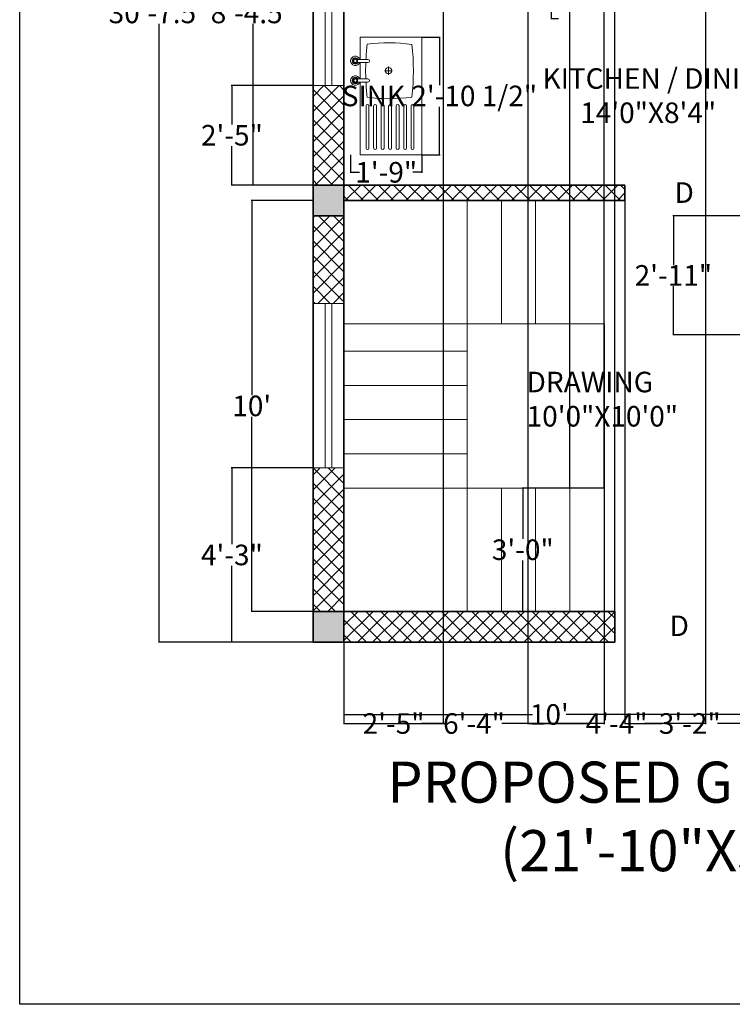
# Model space of a CAD drawing. Units: inches. Extents: x 958 to 1375, y 3152 to 3689.
# Tile 1 of 8: x 958 to 1167, y 3152 to 3440. Entities that reach past the tile are written whole.
import ezdxf

# ---------------------------------------------------------------- set-up
doc = ezdxf.new("R2010")
doc.units = ezdxf.units.IN
doc.header["$MEASUREMENT"] = 0
for name, color, linetype, lineweight in [('A-ANNO-DIMS', 2, 'Continuous', 18), ('A-ANNO-TTLB', 7, 'Continuous', 25), ('A-AREA-IDEN', 7, 'Continuous', 18), ('A-COLS', 7, 'Continuous', 35), ('A-DOOR-IDEN', 7, 'Continuous', 18), ('A-FLOR-CASE', 8, 'Continuous', 25), ('A-FLOR-FIXT', 8, 'Continuous', 18), ('A-FLOR-STRS', 7, 'Continuous', 18), ('A-WALL', 7, 'Continuous', 35), ('windows', 140, 'Continuous', 18)]:
    doc.layers.add(name, color=color, linetype=linetype, lineweight=lineweight)
doc.layers.add('A-COLS-PATT', color=18, linetype='Continuous', lineweight=13, true_color=0x000000)
doc.layers.add('A-WALL-PATT', color=240, linetype='Continuous', lineweight=13, true_color=0xed1f24)
doc.styles.get("Standard").update_dxf_attribs({"font": 'arial.ttf'})
doc.dimstyles.get("Standard").update_dxf_attribs({"dimtxt": 6, "dimasz": 0.18, "dimexe": 0.18, "dimexo": 0.0625, "dimgap": 0.09, "dimtad": 0, "dimtih": 1, "dimtoh": 1, "dimdec": 1, "dimzin": 0, "dimdsep": 46, "dimlunit": 3, "dimtxsty": 'Standard', "dimcen": 0.09, "dimadec": 0, "dimazin": 0, "dimtfac": 1, "dimtdec": 1, "dimtofl": 0, "dimtmove": 0, "dimatfit": 3, "dimfxl": 1, "dimtolj": 1, "dimtzin": 0, "dimarcsym": 0})

# ---------------------------------------------------------------- blocks, each defined once
blk = doc.blocks.new('A$C799204C7')
for p, q in [((0, 34.2), (17.99, 34.2)), ((0, 0), (0, 34.2)), ((2.32, 20.01), (2.32, 32.27)), ((3.13, 20.01), (3.13, 32.27)), ((4.48, 20.01), (4.48, 32.27)), ((5.29, 20.01), (5.29, 32.27)), ((6.64, 20.01), (6.64, 32.27)), ((7.45, 20.01), (7.45, 32.27)), ((8.85, 20.01), (8.85, 32.27)), ((9.66, 20.01), (9.66, 32.27)), ((11.01, 20.01), (11.01, 32.27)), ((11.82, 20.01), (11.82, 32.27)), ((13.22, 20.01), (13.22, 32.27)), ((14.03, 20.01), (14.03, 32.27)), ((15.42, 20.01), (15.42, 32.27)), ((16.24, 20.01), (16.24, 32.27)), ((17.99, 13.08), (17.99, 34.2)), ((18.59, 13.08), (15.71, 13.08)), ((15.71, 12.17), (18.59, 12.17)), ((17.99, 7.36), (17.99, 12.17)), ((8.52, 9.77), (10.9, 9.77)), ((9.73, 11), (9.73, 8.54)), ((18.59, 7.36), (15.71, 7.36)), ((15.71, 6.45), (18.59, 6.45)), ((17.99, 0), (17.99, 6.45)), ((0, 0), (17.99, 0))]:
    blk.add_line(p, q)
for centre, radius in [((19.38, 12.62), 0.684), ((19.38, 12.62), 0.456), ((9.7, 9.77), 0.916), ((19.38, 6.91), 0.684), ((19.38, 6.91), 0.456)]:
    blk.add_circle(centre, radius)
for centre, radius, start, end in [((2.72, 32.27), 0.407, 0, 180), ((4.88, 32.27), 0.407, 0, 180), ((7.05, 32.27), 0.407, 0, 180), ((9.25, 32.27), 0.407, 0, 180), ((11.42, 32.27), 0.407, 0, 180), ((13.62, 32.27), 0.407, 0, 180), ((15.83, 32.27), 0.407, 0, 180), ((2.72, 20.01), 0.407, 180, 0), ((67.33, 9.77), 64.88, 173.1952, 186.8048), ((9.53, -30.19), 48.1, 82.3437, 97.8966), ((4.88, 20.01), 0.407, 180, 0), ((7.05, 20.01), 0.407, 180, 0), ((9.25, 20.01), 0.407, 180, 0), ((11.42, 20.01), 0.407, 180, 0), ((13.62, 20.01), 0.407, 180, 0), ((15.83, 20.01), 0.407, 180, 0), ((-48.51, 9.77), 64.88, 2.9208, 6.8048), ((15.71, 12.62), 0.456, 90, 270), ((-48.51, 9.77), 64.88, 357.8723, 2.115), ((19.38, 12.62), 1.37, 199.6514, 160.3603), ((19.38, 12.62), 0.911, 210.3431, 149.7554), ((15.71, 6.91), 0.456, 90, 270), ((-48.51, 9.77), 64.88, 353.1952, 357.0665), ((19.38, 6.91), 1.37, 199.6514, 160.3603), ((19.38, 6.91), 0.911, 210.3431, 149.7554), ((9.53, 49.73), 48.1, 262.1034, 277.6563)]:
    blk.add_arc(centre, radius, start, end)
blk = doc.blocks.new('*D10')
at = {"layer": 'A-ANNO-DIMS', "color": 0, "lineweight": -2, "transparency": 16777216}
for p, q in [((1053.2, 3257.97), (1053.2, 3236.74)), ((1173.2, 3257.97), (1173.2, 3236.74)), ((1053.38, 3236.92), (1108.3, 3236.92)), ((1173.02, 3236.92), (1118.1, 3236.92))]:
    blk.add_line(p, q, dxfattribs=at)
at = {"layer": 'A-ANNO-DIMS', "color": 0, "transparency": 16777216}
for points in [[(1053.38, 3236.95), (1053.38, 3236.89), (1053.2, 3236.92)], [(1173.02, 3236.95), (1173.02, 3236.89), (1173.2, 3236.92)]]:
    blk.add_solid(points, dxfattribs=at)
at = {"layer": 'Defpoints', "color": 0, "transparency": 16777216}
for p in [(1053.2, 3258.03), (1173.2, 3258.03), (1173.2, 3236.92)]:
    blk.add_point(p, dxfattribs=at)
at = {"layer": 'A-ANNO-DIMS', "color": 0, "transparency": 16777216, "insert": (1113.2, 3236.92), "char_height": 6, "attachment_point": 5}
blk.add_mtext("\\A1;10'", dxfattribs=at)
blk = doc.blocks.new('*D13')
at = {"layer": 'A-ANNO-DIMS', "color": 0, "lineweight": -2, "transparency": 16777216}
for p, q in [((1044.13, 3492.03), (1026.53, 3492.03)), ((1026.71, 3491.85), (1026.71, 3444.94)), ((1026.71, 3391.71), (1026.71, 3438.63)), ((1044.13, 3391.53), (1026.53, 3391.53))]:
    blk.add_line(p, q, dxfattribs=at)
at = {"layer": 'A-ANNO-DIMS', "color": 0, "transparency": 16777216}
for points in [[(1026.68, 3491.85), (1026.74, 3491.85), (1026.71, 3492.03)], [(1026.68, 3391.71), (1026.74, 3391.71), (1026.71, 3391.53)]]:
    blk.add_solid(points, dxfattribs=at)
at = {"layer": 'Defpoints', "color": 0, "transparency": 16777216}
for p in [(1044.2, 3492.03), (1026.71, 3391.53), (1044.2, 3391.53)]:
    blk.add_point(p, dxfattribs=at)
at = {"layer": 'A-ANNO-DIMS', "color": 0, "transparency": 16777216, "insert": (1026.71, 3441.78), "char_height": 6, "attachment_point": 5}
blk.add_mtext('\\A1;8\'-4.5"', dxfattribs=at)
blk = doc.blocks.new('*D14')
at = {"layer": 'A-ANNO-DIMS', "color": 0, "lineweight": -2, "transparency": 16777216}
for p, q in [((1044.13, 3387.03), (1026.06, 3387.03)), ((1026.24, 3386.85), (1026.24, 3330.19)), ((1026.24, 3267.21), (1026.24, 3323.88)), ((1044.13, 3267.03), (1026.06, 3267.03))]:
    blk.add_line(p, q, dxfattribs=at)
at = {"layer": 'A-ANNO-DIMS', "color": 0, "transparency": 16777216}
for points in [[(1026.21, 3386.85), (1026.27, 3386.85), (1026.24, 3387.03)], [(1026.21, 3267.21), (1026.27, 3267.21), (1026.24, 3267.03)]]:
    blk.add_solid(points, dxfattribs=at)
at = {"layer": 'Defpoints', "color": 0, "transparency": 16777216}
for p in [(1044.2, 3387.03), (1026.24, 3267.03), (1044.2, 3267.03)]:
    blk.add_point(p, dxfattribs=at)
at = {"layer": 'A-ANNO-DIMS', "color": 0, "transparency": 16777216, "insert": (1026.24, 3327.03), "char_height": 6, "attachment_point": 5}
blk.add_mtext("\\A1;10'", dxfattribs=at)
blk = doc.blocks.new('*D15')
at = {"layer": 'A-ANNO-DIMS', "color": 0, "lineweight": -2, "transparency": 16777216}
for p, q in [((1044.13, 3625.53), (998.97, 3625.53)), ((999.15, 3625.35), (999.15, 3444.94)), ((999.15, 3258.21), (999.15, 3438.63)), ((1044.13, 3258.03), (998.97, 3258.03))]:
    blk.add_line(p, q, dxfattribs=at)
at = {"layer": 'A-ANNO-DIMS', "color": 0, "transparency": 16777216}
for points in [[(999.12, 3625.35), (999.18, 3625.35), (999.15, 3625.53)], [(999.12, 3258.21), (999.18, 3258.21), (999.15, 3258.03)]]:
    blk.add_solid(points, dxfattribs=at)
at = {"layer": 'Defpoints', "color": 0, "transparency": 16777216}
for p in [(1044.2, 3625.53), (999.15, 3258.03), (1044.2, 3258.03)]:
    blk.add_point(p, dxfattribs=at)
at = {"layer": 'A-ANNO-DIMS', "color": 0, "transparency": 16777216, "insert": (999.15, 3441.78), "char_height": 6, "attachment_point": 5}
blk.add_mtext('\\A1;30\'-7.5"', dxfattribs=at)
blk = doc.blocks.new('WIN-48')
for p, q in [((48, 9), (0, 9)), ((48, 5.5), (0, 5.5)), ((0, 3.5), (48, 3.5)), ((0, 0), (48, 0))]:
    blk.add_line(p, q)
blk = doc.blocks.new('*D32')
at = {"layer": 'A-ANNO-DIMS', "color": 0, "lineweight": -2, "transparency": 16777216}
for p, q in [((1115.92, 3446.28), (1115.92, 3448.44)), ((1116.1, 3448.26), (1129.43, 3448.26)), ((1129.61, 3446.28), (1129.61, 3448.44)), ((1129.61, 3448.26), (1129.79, 3448.26))]:
    blk.add_line(p, q, dxfattribs=at)
at = {"layer": 'A-ANNO-DIMS', "color": 0, "transparency": 16777216}
for points in [[(1116.1, 3448.29), (1116.1, 3448.23), (1115.92, 3448.26)], [(1129.43, 3448.29), (1129.43, 3448.23), (1129.61, 3448.26)]]:
    blk.add_solid(points, dxfattribs=at)
at = {"layer": 'Defpoints', "color": 0, "transparency": 16777216}
for p in [(1129.61, 3448.26), (1115.92, 3446.21), (1129.61, 3446.21)]:
    blk.add_point(p, dxfattribs=at)
at = {"layer": 'A-ANNO-DIMS', "color": 0, "transparency": 16777216, "insert": (1188.42, 3448.26), "char_height": 6, "attachment_point": 5}
blk.add_mtext('\\A1;CHAIR PROFILE 1\'-1 1/2" TYP.', dxfattribs=at)
blk = doc.blocks.new('*D33')
at = {"layer": 'A-ANNO-DIMS', "color": 0, "lineweight": -2, "transparency": 16777216}
for p, q in [((1115.86, 3446.21), (1113.69, 3446.21)), ((1113.87, 3446.21), (1113.87, 3446.39)), ((1113.87, 3446.39), (1114.05, 3446.39)), ((1113.87, 3440.26), (1113.87, 3446.03)), ((1115.86, 3440.08), (1113.69, 3440.08))]:
    blk.add_line(p, q, dxfattribs=at)
at = {"layer": 'A-ANNO-DIMS', "color": 0, "transparency": 16777216}
for points in [[(1113.84, 3446.03), (1113.9, 3446.03), (1113.87, 3446.21)], [(1113.84, 3440.26), (1113.9, 3440.26), (1113.87, 3440.08)]]:
    blk.add_solid(points, dxfattribs=at)
at = {"layer": 'Defpoints', "color": 0, "transparency": 16777216}
for p in [(1113.87, 3446.21), (1115.92, 3446.21), (1115.92, 3440.08)]:
    blk.add_point(p, dxfattribs=at)
at = {"layer": 'A-ANNO-DIMS', "color": 0, "transparency": 16777216, "insert": (1132.43, 3446.39), "char_height": 6, "attachment_point": 5}
blk.add_mtext('\\A1;0\'-6" TYP.', dxfattribs=at)
blk = doc.blocks.new('*D36')
at = {"layer": 'A-ANNO-DIMS', "color": 0, "lineweight": -2, "transparency": 16777216}
for p, q in [((1076.01, 3434.7), (1081.28, 3434.7)), ((1081.1, 3434.52), (1081.1, 3420.73)), ((1081.1, 3400.57), (1081.1, 3414.35)), ((1076.01, 3400.39), (1081.28, 3400.39))]:
    blk.add_line(p, q, dxfattribs=at)
at = {"layer": 'A-ANNO-DIMS', "color": 0, "transparency": 16777216}
for points in [[(1081.07, 3434.52), (1081.13, 3434.52), (1081.1, 3434.7)], [(1081.07, 3400.57), (1081.13, 3400.57), (1081.1, 3400.39)]]:
    blk.add_solid(points, dxfattribs=at)
at = {"layer": 'Defpoints', "color": 0, "transparency": 16777216}
for p in [(1075.95, 3434.7), (1075.95, 3400.39), (1081.1, 3400.39)]:
    blk.add_point(p, dxfattribs=at)
at = {"layer": 'A-ANNO-DIMS', "color": 0, "transparency": 16777216, "insert": (1081.1, 3417.54), "char_height": 6, "attachment_point": 5}
blk.add_mtext('\\A1;SINK 2\'-10 1/2"', dxfattribs=at)
blk = doc.blocks.new('*D37')
at = {"layer": 'A-ANNO-DIMS', "color": 0, "lineweight": -2, "transparency": 16777216}
for p, q in [((1055.14, 3400.32), (1055.14, 3395.06)), ((1075.95, 3400.32), (1075.95, 3395.06)), ((1055.32, 3395.24), (1057.76, 3395.24)), ((1075.77, 3395.24), (1073.33, 3395.24))]:
    blk.add_line(p, q, dxfattribs=at)
at = {"layer": 'A-ANNO-DIMS', "color": 0, "transparency": 16777216}
for points in [[(1055.32, 3395.27), (1055.32, 3395.21), (1055.14, 3395.24)], [(1075.77, 3395.27), (1075.77, 3395.21), (1075.95, 3395.24)]]:
    blk.add_solid(points, dxfattribs=at)
at = {"layer": 'Defpoints', "color": 0, "transparency": 16777216}
for p in [(1055.14, 3400.39), (1075.95, 3400.39), (1055.14, 3395.24)]:
    blk.add_point(p, dxfattribs=at)
at = {"layer": 'A-ANNO-DIMS', "color": 0, "transparency": 16777216, "insert": (1065.54, 3395.24), "char_height": 6, "attachment_point": 5}
blk.add_mtext('\\A1;1\'-9"', dxfattribs=at)
blk = doc.blocks.new('*D38')
at = {"layer": 'A-ANNO-DIMS', "color": 0, "lineweight": -2, "transparency": 16777216}
for p, q in [((1106.9, 3446.15), (1106.9, 3234.1)), ((1158.83, 3446.15), (1158.83, 3234.1)), ((1107.08, 3234.28), (1124.68, 3234.28)), ((1158.65, 3234.28), (1141.05, 3234.28))]:
    blk.add_line(p, q, dxfattribs=at)
at = {"layer": 'A-ANNO-DIMS', "color": 0, "transparency": 16777216}
for points in [[(1107.08, 3234.31), (1107.08, 3234.25), (1106.9, 3234.28)], [(1158.65, 3234.31), (1158.65, 3234.25), (1158.83, 3234.28)]]:
    blk.add_solid(points, dxfattribs=at)
at = {"layer": 'Defpoints', "color": 0, "transparency": 16777216}
for p in [(1106.9, 3446.21), (1158.83, 3446.21), (1158.83, 3234.28)]:
    blk.add_point(p, dxfattribs=at)
at = {"layer": 'A-ANNO-DIMS', "color": 0, "transparency": 16777216, "insert": (1132.86, 3234.28), "char_height": 6, "attachment_point": 5}
blk.add_mtext('\\A1;4\'-4"', dxfattribs=at)
blk = doc.blocks.new('*D40')
at = {"layer": 'A-ANNO-DIMS', "color": 0, "lineweight": -2, "transparency": 16777216}
for p, q in [((1053.2, 3391.47), (1053.2, 3234.1)), ((1082.2, 3391.47), (1082.2, 3234.1)), ((1053.38, 3234.28), (1059.58, 3234.28)), ((1082.02, 3234.28), (1075.81, 3234.28))]:
    blk.add_line(p, q, dxfattribs=at)
at = {"layer": 'A-ANNO-DIMS', "color": 0, "transparency": 16777216}
for points in [[(1053.38, 3234.31), (1053.38, 3234.25), (1053.2, 3234.28)], [(1082.02, 3234.31), (1082.02, 3234.25), (1082.2, 3234.28)]]:
    blk.add_solid(points, dxfattribs=at)
at = {"layer": 'Defpoints', "color": 0, "transparency": 16777216}
for p in [(1053.2, 3391.53), (1082.2, 3391.53), (1082.2, 3234.28)]:
    blk.add_point(p, dxfattribs=at)
at = {"layer": 'A-ANNO-DIMS', "color": 0, "transparency": 16777216, "insert": (1067.7, 3234.28), "char_height": 6, "attachment_point": 5}
blk.add_mtext('\\A1;2\'-5"', dxfattribs=at)
blk = doc.blocks.new('*D41')
at = {"layer": 'A-ANNO-DIMS', "color": 0, "lineweight": -2, "transparency": 16777216}
for p, q in [((1129.13, 3303.03), (1105.27, 3303.03)), ((1105.45, 3302.85), (1105.45, 3288.19)), ((1105.45, 3267.21), (1105.45, 3281.88)), ((1129.13, 3267.03), (1105.27, 3267.03))]:
    blk.add_line(p, q, dxfattribs=at)
at = {"layer": 'A-ANNO-DIMS', "color": 0, "transparency": 16777216}
for points in [[(1105.42, 3302.85), (1105.48, 3302.85), (1105.45, 3303.03)], [(1105.42, 3267.21), (1105.48, 3267.21), (1105.45, 3267.03)]]:
    blk.add_solid(points, dxfattribs=at)
at = {"layer": 'Defpoints', "color": 0, "transparency": 16777216}
for p in [(1105.45, 3303.03), (1129.2, 3303.03), (1129.2, 3267.03)]:
    blk.add_point(p, dxfattribs=at)
at = {"layer": 'A-ANNO-DIMS', "color": 0, "transparency": 16777216, "insert": (1105.45, 3285.03), "char_height": 6, "attachment_point": 5}
blk.add_mtext('\\A1;3\'-0"', dxfattribs=at)
blk = doc.blocks.new('*D42')
at = {"layer": 'A-ANNO-DIMS', "color": 0, "lineweight": -2, "transparency": 16777216}
for p, q in [((1053.2, 3350.97), (1053.2, 3234.1)), ((1129.2, 3350.97), (1129.2, 3234.1)), ((1053.38, 3234.28), (1083.12, 3234.28)), ((1129.02, 3234.28), (1099.28, 3234.28))]:
    blk.add_line(p, q, dxfattribs=at)
at = {"layer": 'A-ANNO-DIMS', "color": 0, "transparency": 16777216}
for points in [[(1053.38, 3234.31), (1053.38, 3234.25), (1053.2, 3234.28)], [(1129.02, 3234.31), (1129.02, 3234.25), (1129.2, 3234.28)]]:
    blk.add_solid(points, dxfattribs=at)
at = {"layer": 'Defpoints', "color": 0, "transparency": 16777216}
for p in [(1053.2, 3351.03), (1129.2, 3351.03), (1129.2, 3234.28)]:
    blk.add_point(p, dxfattribs=at)
at = {"layer": 'A-ANNO-DIMS', "color": 0, "transparency": 16777216, "insert": (1091.2, 3234.28), "char_height": 6, "attachment_point": 5}
blk.add_mtext('\\A1;6\'-4"', dxfattribs=at)
blk = doc.blocks.new('*D43')
at = {"layer": 'A-ANNO-DIMS', "color": 0, "lineweight": -2, "transparency": 16777216}
for p, q in [((1119.2, 3303.1), (1119.2, 3649.46)), ((1119.38, 3649.28), (1129.02, 3649.28)), ((1129.2, 3303.1), (1129.2, 3649.46)), ((1129.2, 3649.28), (1129.38, 3649.28))]:
    blk.add_line(p, q, dxfattribs=at)
at = {"layer": 'A-ANNO-DIMS', "color": 0, "transparency": 16777216}
for points in [[(1119.38, 3649.31), (1119.38, 3649.25), (1119.2, 3649.28)], [(1129.02, 3649.31), (1129.02, 3649.25), (1129.2, 3649.28)]]:
    blk.add_solid(points, dxfattribs=at)
at = {"layer": 'Defpoints', "color": 0, "transparency": 16777216}
for p in [(1129.2, 3649.28), (1119.2, 3303.03), (1129.2, 3303.03)]:
    blk.add_point(p, dxfattribs=at)
at = {"layer": 'A-ANNO-DIMS', "color": 0, "transparency": 16777216, "insert": (1139.77, 3649.28), "char_height": 6, "attachment_point": 5}
blk.add_mtext('\\A1;0\'-10"', dxfattribs=at)
blk = doc.blocks.new('*D44')
at = {"layer": 'A-ANNO-DIMS', "color": 0, "lineweight": -2, "transparency": 16777216}
for p, q in [((1132.32, 3267.1), (1132.32, 3649.46)), ((1132.5, 3649.28), (1144.69, 3649.28)), ((1173.02, 3649.28), (1160.82, 3649.28)), ((1173.2, 3267.1), (1173.2, 3649.46))]:
    blk.add_line(p, q, dxfattribs=at)
at = {"layer": 'A-ANNO-DIMS', "color": 0, "transparency": 16777216}
for points in [[(1132.5, 3649.31), (1132.5, 3649.25), (1132.32, 3649.28)], [(1173.02, 3649.31), (1173.02, 3649.25), (1173.2, 3649.28)]]:
    blk.add_solid(points, dxfattribs=at)
at = {"layer": 'Defpoints', "color": 0, "transparency": 16777216}
for p in [(1173.2, 3649.28), (1132.32, 3267.03), (1173.2, 3267.03)]:
    blk.add_point(p, dxfattribs=at)
at = {"layer": 'A-ANNO-DIMS', "color": 0, "transparency": 16777216, "insert": (1152.76, 3649.28), "char_height": 6, "attachment_point": 5}
blk.add_mtext('\\A1;3\'-5"', dxfattribs=at)
blk = doc.blocks.new('*D45')
at = {"layer": 'A-ANNO-DIMS', "color": 0, "lineweight": -2, "transparency": 16777216}
for p, q in [((1173.13, 3382.53), (1149.27, 3382.53)), ((1149.45, 3382.35), (1149.45, 3368.24)), ((1149.45, 3347.92), (1149.45, 3362.04)), ((1173.13, 3347.74), (1149.27, 3347.74))]:
    blk.add_line(p, q, dxfattribs=at)
at = {"layer": 'A-ANNO-DIMS', "color": 0, "transparency": 16777216}
for points in [[(1149.42, 3382.35), (1149.48, 3382.35), (1149.45, 3382.53)], [(1149.42, 3347.92), (1149.48, 3347.92), (1149.45, 3347.74)]]:
    blk.add_solid(points, dxfattribs=at)
at = {"layer": 'Defpoints', "color": 0, "transparency": 16777216}
for p in [(1149.45, 3382.53), (1173.2, 3382.53), (1173.2, 3347.74)]:
    blk.add_point(p, dxfattribs=at)
at = {"layer": 'A-ANNO-DIMS', "color": 0, "transparency": 16777216, "insert": (1149.45, 3365.14), "char_height": 6, "attachment_point": 5}
blk.add_mtext('\\A1;2\'-11"', dxfattribs=at)
blk = doc.blocks.new('*D56')
at = {"layer": 'A-ANNO-DIMS', "color": 0, "lineweight": -2, "transparency": 16777216}
for p, q in [((1044.13, 3308.96), (1020.27, 3308.96)), ((1020.45, 3308.78), (1020.45, 3286.65)), ((1020.45, 3258.21), (1020.45, 3280.34)), ((1044.13, 3258.03), (1020.27, 3258.03))]:
    blk.add_line(p, q, dxfattribs=at)
at = {"layer": 'A-ANNO-DIMS', "color": 0, "transparency": 16777216}
for points in [[(1020.42, 3308.78), (1020.48, 3308.78), (1020.45, 3308.96)], [(1020.42, 3258.21), (1020.48, 3258.21), (1020.45, 3258.03)]]:
    blk.add_solid(points, dxfattribs=at)
at = {"layer": 'Defpoints', "color": 0, "transparency": 16777216}
for p in [(1020.45, 3308.96), (1044.2, 3308.96), (1044.2, 3258.03)]:
    blk.add_point(p, dxfattribs=at)
at = {"layer": 'A-ANNO-DIMS', "color": 0, "transparency": 16777216, "insert": (1020.45, 3283.5), "char_height": 6, "attachment_point": 5}
blk.add_mtext('\\A1;4\'-3"', dxfattribs=at)
blk = doc.blocks.new('*D57')
at = {"layer": 'A-ANNO-DIMS', "color": 0, "lineweight": -2, "transparency": 16777216}
for p, q in [((1044.13, 3420.58), (1020.27, 3420.58)), ((1020.45, 3420.4), (1020.45, 3409.21)), ((1020.45, 3391.71), (1020.45, 3402.9)), ((1044.13, 3391.53), (1020.27, 3391.53))]:
    blk.add_line(p, q, dxfattribs=at)
at = {"layer": 'A-ANNO-DIMS', "color": 0, "transparency": 16777216}
for points in [[(1020.42, 3420.4), (1020.48, 3420.4), (1020.45, 3420.58)], [(1020.42, 3391.71), (1020.48, 3391.71), (1020.45, 3391.53)]]:
    blk.add_solid(points, dxfattribs=at)
at = {"layer": 'Defpoints', "color": 0, "transparency": 16777216}
for p in [(1020.45, 3420.58), (1044.2, 3420.58), (1044.2, 3391.53)]:
    blk.add_point(p, dxfattribs=at)
at = {"layer": 'A-ANNO-DIMS', "color": 0, "transparency": 16777216, "insert": (1020.45, 3406.06), "char_height": 6, "attachment_point": 5}
blk.add_mtext('\\A1;2\'-5"', dxfattribs=at)
blk = doc.blocks.new('*D60')
at = {"layer": 'A-ANNO-DIMS', "color": 0, "lineweight": -2, "transparency": 16777216}
for p, q in [((1135.31, 3386.97), (1135.31, 3234.1)), ((1173.2, 3386.97), (1173.2, 3234.1)), ((1135.49, 3234.28), (1146.19, 3234.28)), ((1173.02, 3234.28), (1162.32, 3234.28))]:
    blk.add_line(p, q, dxfattribs=at)
at = {"layer": 'A-ANNO-DIMS', "color": 0, "transparency": 16777216}
for points in [[(1135.49, 3234.31), (1135.49, 3234.25), (1135.31, 3234.28)], [(1173.02, 3234.31), (1173.02, 3234.25), (1173.2, 3234.28)]]:
    blk.add_solid(points, dxfattribs=at)
at = {"layer": 'Defpoints', "color": 0, "transparency": 16777216}
for p in [(1135.31, 3387.03), (1173.2, 3387.03), (1173.2, 3234.28)]:
    blk.add_point(p, dxfattribs=at)
at = {"layer": 'A-ANNO-DIMS', "color": 0, "transparency": 16777216, "insert": (1154.25, 3234.28), "char_height": 6, "attachment_point": 5}
blk.add_mtext('\\A1;3\'-2"', dxfattribs=at)

msp = doc.modelspace()

# ---------------------------------------------------------------- hatches: boundary and pattern name
at = {"layer": 'A-COLS-PATT'}
h = msp.add_hatch(color=256, dxfattribs=at)
h.dxf.hatch_style = 1
h.paths.add_polyline_path([(1053.2, 3625.53), (1044.2, 3625.53), (1044.2, 3616.53), (1053.2, 3616.53)])
h.paths.add_polyline_path([(1182.2, 3625.53), (1173.2, 3625.53), (1173.2, 3616.53), (1182.2, 3616.53)])
h.paths.add_polyline_path([(1306.7, 3625.53), (1297.7, 3625.53), (1297.7, 3616.53), (1306.7, 3616.53)])
h.paths.add_polyline_path([(1306.7, 3501.03), (1297.7, 3501.03), (1297.7, 3492.03), (1306.7, 3492.03)])
h.paths.add_polyline_path([(1306.7, 3391.53), (1297.7, 3391.53), (1297.7, 3382.53), (1306.7, 3382.53)])
h.paths.add_polyline_path([(1306.7, 3267.03), (1297.7, 3267.03), (1297.7, 3258.03), (1306.7, 3258.03)])
h.paths.add_polyline_path([(1182.2, 3267.03), (1173.2, 3267.03), (1173.2, 3258.03), (1182.2, 3258.03)])
h.paths.add_polyline_path([(1053.2, 3267.03), (1044.2, 3267.03), (1044.2, 3258.03), (1053.2, 3258.03)])
h.paths.add_polyline_path([(1053.2, 3391.53), (1044.2, 3391.53), (1044.2, 3382.53), (1053.2, 3382.53)])
h.paths.add_polyline_path([(1053.2, 3501.03), (1044.2, 3501.03), (1044.2, 3492.03), (1053.2, 3492.03)])
h.paths.add_polyline_path([(1182.2, 3501.03), (1173.2, 3501.03), (1173.2, 3492.03), (1182.2, 3492.03)])
h.paths.add_polyline_path([(1182.2, 3391.53), (1173.2, 3391.53), (1173.2, 3382.53), (1182.2, 3382.53)])
at = {"layer": 'A-WALL-PATT'}
h = msp.add_hatch(dxfattribs=at)
h.set_pattern_fill('ANSI37', color=256, scale=25)
h.paths.add_polyline_path([(1080.68, 3625.53), (1053.2, 3625.53), (1053.2, 3616.53), (1080.68, 3616.53)])
h.paths.add_polyline_path([(1053.2, 3616.53), (1044.2, 3616.53), (1044.2, 3587.05), (1053.2, 3587.05)])
h.paths.add_polyline_path([(1173.2, 3625.53), (1128.68, 3625.53), (1128.68, 3616.53), (1173.2, 3616.53)])
h.paths.add_polyline_path([(1215.78, 3625.53), (1182.2, 3625.53), (1182.2, 3616.53), (1215.78, 3616.53)])
h.paths.add_polyline_path([(1297.7, 3625.53), (1263.78, 3625.53), (1263.78, 3616.53), (1297.7, 3616.53)])
h.paths.add_polyline_path([(1177.7, 3616.53), (1173.2, 3616.53), (1173.2, 3501.03), (1177.7, 3501.03)])
h.paths.add_polyline_path([(1053.2, 3539.05), (1044.2, 3539.05), (1044.2, 3501.03), (1053.2, 3501.03)])
h.paths.add_polyline_path([(1135.44, 3496.53), (1053.2, 3496.53), (1053.2, 3492.03), (1135.44, 3492.03)])
h.paths.add_polyline_path([(1306.7, 3616.53), (1297.7, 3616.53), (1297.7, 3586.38), (1306.7, 3586.38)])
h.paths.add_polyline_path([(1306.7, 3538.38), (1297.7, 3538.38), (1297.7, 3501.03), (1306.7, 3501.03)])
h.paths.add_polyline_path([(1297.7, 3496.53), (1216.84, 3496.53), (1216.84, 3492.03), (1297.7, 3492.03)])
h.paths.add_polyline_path([(1306.7, 3492.03), (1297.7, 3492.03), (1297.7, 3481.63), (1306.7, 3481.63)])
h.paths.add_polyline_path([(1306.7, 3457.63), (1297.7, 3457.63), (1297.7, 3444.03), (1225.7, 3444.03), (1225.7, 3462.51), (1221.2, 3462.51), (1221.2, 3391.53), (1182.2, 3391.53), (1182.2, 3387.03), (1225.7, 3387.03), (1225.7, 3439.53), (1297.7, 3439.53), (1297.7, 3428.57), (1306.7, 3428.57)])
h.paths.add_polyline_path([(1306.7, 3404.57), (1297.7, 3404.57), (1297.7, 3391.53), (1306.7, 3391.53)], flags=17)
h.paths.add_polyline_path([(1297.7, 3391.53), (1253.12, 3391.53), (1253.12, 3387.03), (1297.7, 3387.03)], flags=17)
h.paths.add_polyline_path([(1306.7, 3382.53), (1297.7, 3382.53), (1297.7, 3354.01), (1306.7, 3354.01)])
h.paths.add_polyline_path([(1306.7, 3306.01), (1297.7, 3306.01), (1297.7, 3267.03), (1306.7, 3267.03)])
h.paths.add_polyline_path([(1297.7, 3267.03), (1254.05, 3267.03), (1254.05, 3258.03), (1297.7, 3258.03)])
h.paths.add_polyline_path([(1177.7, 3347.74), (1173.2, 3347.74), (1173.2, 3267.03), (1177.7, 3267.03)])
h.paths.add_polyline_path([(1206.05, 3267.03), (1182.2, 3267.03), (1182.2, 3258.03), (1206.05, 3258.03)])
h.paths.add_polyline_path([(1053.2, 3308.96), (1044.2, 3308.96), (1044.2, 3267.03), (1053.2, 3267.03)])
h.paths.add_polyline_path([(1053.2, 3382.53), (1044.2, 3382.53), (1044.2, 3356.96), (1053.2, 3356.96)])
h.paths.add_polyline_path([(1053.2, 3420.58), (1044.2, 3420.58), (1044.2, 3391.53), (1053.2, 3391.53)])
h.paths.add_polyline_path([(1053.2, 3492.03), (1044.2, 3492.03), (1044.2, 3468.58), (1053.2, 3468.58)])
h = msp.add_hatch(dxfattribs=at)
h.set_pattern_fill('ANSI37', color=256, scale=25)
h.paths.add_polyline_path([(1135.31, 3391.53), (1053.2, 3391.53), (1053.2, 3387.03), (1135.31, 3387.03)])
h = msp.add_hatch(dxfattribs=at)
h.set_pattern_fill('ANSI37', color=256, scale=25)
h.paths.add_polyline_path([(1132.32, 3267.03), (1053.2, 3267.03), (1053.2, 3258.03), (1132.32, 3258.03)])

# ---------------------------------------------------------------- linework, layer by layer
at = {"layer": 'A-ANNO-TTLB'}
msp.add_lwpolyline([(958.44, 3689.37), (1374.91, 3689.37), (1374.91, 3152.28), (958.44, 3152.28)], close=True, dxfattribs=at)
at = {"layer": 'A-COLS'}
for p, q in [((1044.2, 3391.53), (1053.2, 3391.53)), ((1044.2, 3382.53), (1044.2, 3391.53)), ((1053.2, 3391.53), (1053.2, 3382.53)), ((1053.2, 3382.53), (1044.2, 3382.53))]:
    msp.add_line(p, q, dxfattribs=at)
at = {"layer": 'A-FLOR-CASE'}
msp.add_line((1082.2, 3492.03), (1082.2, 3391.53), dxfattribs=at)
at = {"layer": 'A-FLOR-STRS'}
for p, q in [((1053.2, 3387.03), (1053.2, 3351.03)), ((1089.2, 3267.03), (1089.2, 3387.03)), ((1099.2, 3351.03), (1099.2, 3387.03)), ((1109.2, 3351.03), (1109.2, 3387.03)), ((1119.2, 3351.03), (1119.2, 3387.03)), ((1129.2, 3351.03), (1129.2, 3387.03)), ((1053.2, 3351.03), (1129.2, 3351.03)), ((1053.2, 3343.03), (1089.2, 3343.03)), ((1053.2, 3333.03), (1089.2, 3333.03)), ((1053.2, 3323.03), (1089.2, 3323.03)), ((1053.2, 3313.03), (1089.2, 3313.03)), ((1053.2, 3267.03), (1053.2, 3303.03)), ((1053.2, 3303.03), (1129.2, 3303.03)), ((1099.2, 3267.03), (1099.2, 3303.03)), ((1109.2, 3267.03), (1109.2, 3303.03)), ((1119.2, 3267.03), (1119.2, 3303.03)), ((1129.2, 3267.03), (1129.2, 3303.03)), ((1053.2, 3267.03), (1053.2, 3267.03)), ((1053.2, 3267.03), (1089.2, 3267.03))]:
    msp.add_line(p, q, dxfattribs=at)
at = {"layer": 'A-WALL'}
for p, q in [((1044.2, 3625.53), (1044.2, 3258.03)), ((1053.2, 3625.53), (1053.2, 3258.03)), ((1044.2, 3391.53), (1135.31, 3391.53)), ((1135.31, 3391.53), (1135.31, 3387.03)), ((1053.2, 3387.03), (1135.31, 3387.03)), ((1044.2, 3267.03), (1132.32, 3267.03)), ((1132.32, 3267.03), (1132.32, 3258.03)), ((1044.2, 3258.03), (1132.32, 3258.03))]:
    msp.add_line(p, q, dxfattribs=at)
at = {"layer": 'windows'}
for p, q in [((1053.2, 3420.58), (1044.2, 3420.58)), ((1044.2, 3356.96), (1053.2, 3356.96)), ((1053.2, 3308.96), (1044.2, 3308.96))]:
    msp.add_line(p, q, dxfattribs=at)

# ---------------------------------------------------------------- block references
at = {"layer": 'A-FLOR-FIXT', "xscale": 1.0032, "yscale": 1.0032, "zscale": 1.0032, "rotation": 180}
msp.add_blockref('A$C799204C7', (1075.95, 3434.7), dxfattribs=at)
at = {"layer": 'windows', "rotation": 90}
for p in [(1053.2, 3420.58), (1053.2, 3308.96)]:
    msp.add_blockref('WIN-48', p, dxfattribs=at)

# ---------------------------------------------------------------- texts
at = {"layer": 'A-ANNO-TTLB', "insert": (1065.83, 3223.15), "char_height": 12, "attachment_point": 1}
msp.add_mtext_dynamic_manual_height_columns('PROPOSED G - FLOOR PLAN\\P         (21\'-10"X30\'-6")', width=421.2695, gutter_width=1, heights=[0], dxfattribs=at)
at = {"layer": 'A-AREA-IDEN', "char_height": 6, "attachment_point": 1}
for s, width, insert in [('KITCHEN / DINING\\P      14\'0"X8\'4"', 114.4555, (1111.24, 3425.63)), ('DRAWING\\P10\'0"X10\'0"', 59.9342, (1106.57, 3337))]:
    msp.add_mtext_dynamic_manual_height_columns(s, width=width, gutter_width=1, heights=[0], dxfattribs=dict(at, insert=insert))
at = {"layer": 'A-DOOR-IDEN', "char_height": 6, "attachment_point": 1}
for insert in [(1149.81, 3392.32), (1149.81, 3392.32), (1148.36, 3265.82)]:
    msp.add_mtext_dynamic_manual_height_columns('D ', width=17.9455, gutter_width=1, heights=[0], dxfattribs=dict(at, insert=insert))

# ---------------------------------------------------------------- dimensions: what is measured, and where the dimension line sits
at = {"layer": 'A-ANNO-DIMS'}
for base, p1, p2, override, picture, middle in [((1129.2, 3649.28), (1119.2, 3303.03), (1129.2, 3303.03), {"dimdec": 1, "dimlfac": 1, "dimrnd": 0, "dimzin": 1, "dimdsep": 46, "dimlunit": 4, "dimfrac": 2}, '*D43', (1139.77, 3649.28)), ((1173.2, 3649.28), (1132.32, 3267.03), (1173.2, 3267.03), {"dimdec": 1, "dimlfac": 1, "dimrnd": 0, "dimzin": 1, "dimdsep": 46, "dimlunit": 4, "dimfrac": 2}, '*D44', (1152.76, 3649.28)), ((1158.83, 3234.28), (1106.9, 3446.21), (1158.83, 3446.21), {"dimdec": 1, "dimlfac": 1, "dimrnd": 0, "dimzin": 1, "dimdsep": 46, "dimlunit": 4, "dimfrac": 2}, '*D38', (1132.86, 3234.28)), ((1082.2, 3234.28), (1053.2, 3391.53), (1082.2, 3391.53), {"dimdec": 1, "dimlfac": 1, "dimrnd": 0, "dimzin": 1, "dimdsep": 46, "dimlunit": 4, "dimfrac": 2}, '*D40', (1067.7, 3234.28)), ((1173.2, 3234.28), (1135.31, 3387.03), (1173.2, 3387.03), {"dimdec": 1, "dimlfac": 1, "dimrnd": 0, "dimzin": 1, "dimdsep": 46, "dimlunit": 4, "dimfrac": 2}, '*D60', (1154.25, 3234.28)), ((1129.2, 3234.28), (1053.2, 3351.03), (1129.2, 3351.03), {"dimdec": 1, "dimlfac": 1, "dimrnd": 0, "dimzin": 1, "dimdsep": 46, "dimlunit": 4, "dimfrac": 2}, '*D42', (1091.2, 3234.28)), ((1173.2, 3236.92), (1053.2, 3258.03), (1173.2, 3258.03), {"dimclrd": 0, "dimclre": 0, "dimclrt": 0}, '*D10', (1113.2, 3236.92))]:
    dim = msp.add_linear_dim(base=base, p1=p1, p2=p2, dimstyle='Standard', override=override, dxfattribs=at)
    dim.commit()
    dim.dimension.update_dxf_attribs({"geometry": picture, "text_midpoint": middle})
for base, p1, p2, angle, override, picture, middle in [((999.15, 3258.03), (1044.2, 3625.53), (1044.2, 3258.03), 90, {"dimclrd": 0, "dimclre": 0, "dimclrt": 0}, '*D15', (999.15, 3441.78)), ((1026.71, 3391.53), (1044.2, 3492.03), (1044.2, 3391.53), 90, {"dimclrd": 0, "dimclre": 0, "dimclrt": 0}, '*D13', (1026.71, 3441.78)), ((1020.4472, 3420.5785), (1044.1972, 3391.5349), (1044.1972, 3420.5785), 90, {"dimdec": 1, "dimlfac": 1, "dimrnd": 0, "dimzin": 1, "dimdsep": 46, "dimlunit": 4, "dimfrac": 2}, '*D57', (1020.4472, 3406.0567)), ((1055.14, 3395.24), (1075.95, 3400.39), (1055.14, 3400.39), 180, {"dimdec": 1, "dimlfac": 1, "dimrnd": 0, "dimzin": 1, "dimdsep": 46, "dimlunit": 4, "dimfrac": 2}, '*D37', (1065.54, 3395.24)), ((1026.24, 3267.03), (1044.2, 3387.03), (1044.2, 3267.03), 90, {"dimclrd": 0, "dimclre": 0, "dimclrt": 0}, '*D14', (1026.24, 3327.03)), ((1149.45, 3382.53), (1173.2, 3347.74), (1173.2, 3382.53), 90, {"dimdec": 1, "dimlfac": 1, "dimrnd": 0, "dimzin": 1, "dimdsep": 46, "dimlunit": 4, "dimfrac": 2}, '*D45', (1149.45, 3365.14)), ((1020.45, 3308.96), (1044.2, 3258.03), (1044.2, 3308.96), 90, {"dimdec": 1, "dimlfac": 1, "dimrnd": 0, "dimzin": 1, "dimdsep": 46, "dimlunit": 4, "dimfrac": 2}, '*D56', (1020.45, 3283.5)), ((1105.45, 3303.03), (1129.2, 3267.03), (1129.2, 3303.03), 90, {"dimdec": 1, "dimlfac": 1, "dimrnd": 0, "dimzin": 1, "dimdsep": 46, "dimlunit": 4, "dimfrac": 2}, '*D41', (1105.45, 3285.03))]:
    dim = msp.add_linear_dim(base=base, p1=p1, p2=p2, angle=angle, dimstyle='Standard', override=override, dxfattribs=at)
    dim.commit()
    dim.dimension.update_dxf_attribs({"geometry": picture, "text_midpoint": middle})
dim = msp.add_linear_dim(base=(1129.61, 3448.26), p1=(1115.92, 3446.21), p2=(1129.61, 3446.21), text='CHAIR PROFILE <> TYP.', dimstyle='Standard', override={"dimdec": 1, "dimlfac": 1, "dimrnd": 0, "dimzin": 1, "dimdsep": 46, "dimlunit": 4, "dimfrac": 2}, dxfattribs=at)
dim.commit()
dim.dimension.update_dxf_attribs({"geometry": '*D32', "text_midpoint": (1188.42, 3448.26)})
for base, p1, p2, angle, text, picture, middle in [((1113.87, 3446.21), (1115.92, 3440.08), (1115.92, 3446.21), 90, '<> TYP.', '*D33', (1132.43, 3446.39)), ((1081.1, 3400.39), (1075.95, 3434.7), (1075.95, 3400.39), 270, 'SINK <>', '*D36', (1081.1, 3417.54))]:
    dim = msp.add_linear_dim(base=base, p1=p1, p2=p2, angle=angle, text=text, dimstyle='Standard', override={"dimdec": 1, "dimlfac": 1, "dimrnd": 0, "dimzin": 1, "dimdsep": 46, "dimlunit": 4, "dimfrac": 2}, dxfattribs=at)
    dim.commit()
    dim.dimension.update_dxf_attribs({"geometry": picture, "text_midpoint": middle})

doc.saveas('drawing.dxf')
